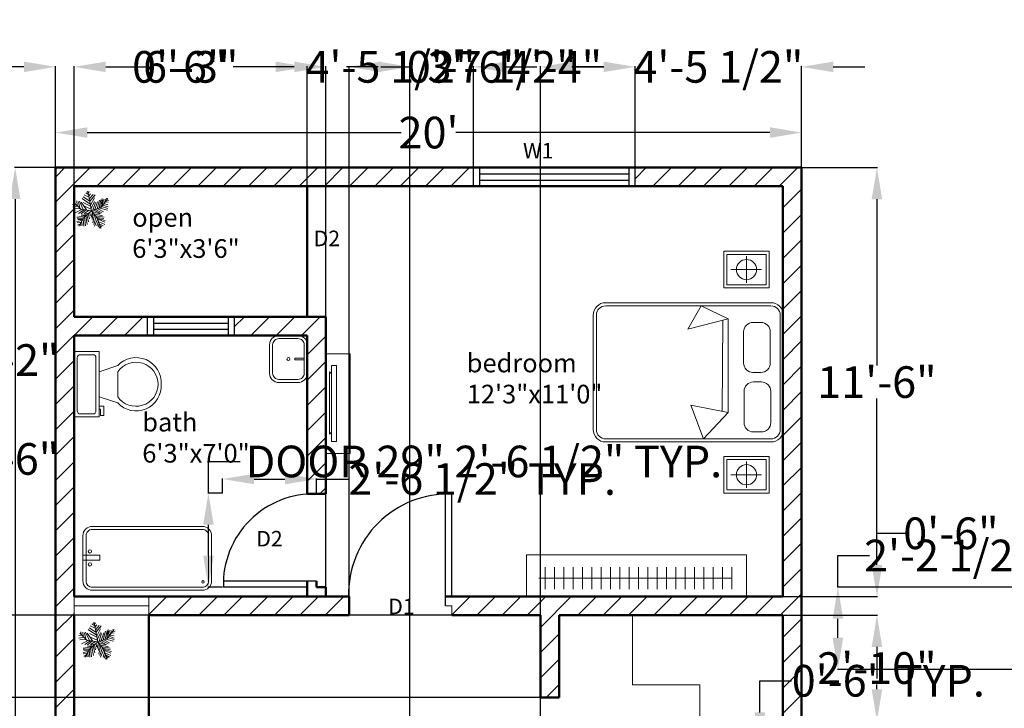
# Model space of a CAD drawing. Units: inches. Extents: x 21 to 3450, y 4 to 2137.
# Tile 11 of 14: x 2805 to 3122, y 1333 to 1554. Entities that reach past the tile are written whole.
import ezdxf

# ---------------------------------------------------------------- set-up
doc = ezdxf.new("R2010")
doc.units = ezdxf.units.IN
doc.header["$MEASUREMENT"] = 0
for name, color, linetype, lineweight in [('A-ANNO-DIMS', 2, 'Continuous', 18), ('A-ANNO-TEXT', 7, 'Continuous', 18), ('A-AREA-IDEN', 3, 'Continuous', 18), ('A-DOOR', 4, 'Continuous', 25), ('A-FLOR-FIXT', 9, 'Continuous', 18), ('A-FURN', 8, 'Continuous', 18), ('A-GLAZ', 3, 'Continuous', 25), ('A-WALL', 7, 'Continuous', 50), ('A-WALL-PATT', 8, 'Continuous', 13), ('L-PLNT', 94, 'Continuous', 13)]:
    doc.layers.add(name, color=color, linetype=linetype, lineweight=lineweight)
doc.styles.get("Standard").update_dxf_attribs({"font": 'arial.ttf'})
doc.dimstyles.get("Standard").update_dxf_attribs({"dimtxt": 10.18, "dimasz": 10.18, "dimexe": 0.18, "dimexo": 0.0625, "dimgap": 0.09, "dimtad": 0, "dimtih": 1, "dimtoh": 1, "dimdec": 0, "dimzin": 0, "dimdsep": 46, "dimlunit": 3, "dimtxsty": 'Standard', "dimcen": 0.09, "dimadec": 0, "dimazin": 0, "dimtfac": 1, "dimtdec": 0, "dimtofl": 0, "dimtmove": 0, "dimatfit": 3, "dimfxl": 1, "dimtolj": 1, "dimtzin": 0, "dimarcsym": 0})

# ---------------------------------------------------------------- blocks, each defined once
blk = doc.blocks.new('*U4')
for p, q in [((9.5, -6), (9.5, -2)), ((-10, -8.5), (-8, -8.5)), ((-10, -9.5), (-10, -8.5)), ((-7, -9.5), (-10, -9.5)), ((-8, -8.5), (-8, -8)), ((-7, -8), (-7, -9.5)), ((-4, -8), (-6, -14)), ((4, -8), (6, -14)), ((4, -14), (-4, -14))]:
    blk.add_line(p, q)
blk.add_lwpolyline([(10.5, -8), (10.5, 0), (-10.5, 0), (-10.5, -8)], close=True)
for points in [[(-9.5, -2), (-9.5, -6)], [(8.5, -1), (-8.5, -1)], [(-8.5, -7), (8.5, -7)]]:
    blk.add_lwpolyline(points)
for centre, radius, start, end in [((-8.625, -1.875), 0.8839, 81.8699, 188.1301), ((8.625, -1.875), 0.8839, 351.8699, 98.1301), ((-8.625, -6.125), 0.8839, 171.869898, 278.1301), ((8.625, -6.125), 0.8839, 261.8699, 8.1301), ((-0.4772, -19.9188), 8.0953, 133.01722, 273.38), ((0.0374, -19.8731), 7.127, 124.50543, 269.7), ((-0.0373, -19.8731), 7.127, 270.3, 55.4946), ((0.4773, -19.9188), 8.0953, 266.62, 46.9828)]:
    blk.add_arc(centre, radius, start, end)
blk = doc.blocks.new('*U6')
for p, q in [((-48.585, 21.131), (-49.309, 29.026)), ((-3.665, 19.273), (-27.574, 35.527)), ((-5.114, 28.097), (-24.676, 40.636)), ((-7.288, 39.707), (-21.778, 46.673)), ((-8.737, 47.138), (-17.069, 52.711)), ((-10.186, 53.64), (-13.084, 55.962)), ((0, 0), (-10.5, 57)), ((-9.099, 51.782), (-6.563, 55.962)), ((-7.65, 43.423), (-2.578, 49.46)), ((-5.839, 35.992), (4.667, 48.067)), ((-5.114, 27.632), (10.463, 46.673)), ((-2.941, 16.486), (8.652, 37.85)), ((16.259, 5.805), (23.142, 31.348)), ((22.055, 7.198), (27.489, 32.277)), ((27, 9), (48, 36)), ((27.127, 9.056), (31.112, 35.992)), ((31.836, 30.883), (32.561, 16.486)), ((35.096, 32.741), (37.27, 22.524)), ((38.719, 34.134), (41.979, 28.561)), ((43.791, 29.954), (51.036, 30.883)), ((44.153, 36.456), (45.239, 32.741)), ((-47.498, 19.737), (-55.83, 18.344)), ((-40.615, 13.7), (-55.105, 10.913)), ((-31.5, 4.5), (-52.5, 25.5)), ((-33.37, 6.269), (-52.207, 5.34)), ((-28.299, 3.483), (-47.86, -5.805)), ((-43.513, 28.561), (-42.427, 15.558)), ((-38.442, 26.239), (-34.819, 7.663)), ((-21.416, 3.018), (-38.079, -8.128)), ((-35.544, 28.097), (-24.314, 3.947)), ((0, 0), (-31.5, 4.5)), ((-14.533, 2.09), (-30.834, 25.31)), ((-15.982, 2.09), (-30.11, -9.521)), ((-24.314, 23.917), (-2.941, 13.7)), ((0, 0), (-22.5, -19.5)), ((-6.563, 1.161), (-21.416, -8.128)), ((-20.691, 13.7), (-1.129, 4.876)), ((-1.129, 6.734), (9.014, 26.704)), ((0, 0), (27, 9)), ((0, 0), (18, -22.5)), ((3.942, 1.625), (11.187, 24.381)), ((6.478, 1.625), (26.04, -8.592)), ((10.101, 3.483), (17.708, 26.239)), ((11.187, 3.483), (30.749, -5.805)), ((18.07, 5.805), (35.096, -3.483)), ((24.229, 7.663), (46.688, 1.625)), ((29.662, 12.307), (48.137, 6.269)), ((33.285, 16.486), (48.862, 10.913)), ((36.183, 19.737), (48.137, 17.88)), ((40.53, 25.775), (48.862, 24.846)), ((-17.431, -15.094), (-42.789, -18.809)), ((-24.314, -21.596), (-42.427, -22.06)), ((-26.849, -26.24), (-40.253, -25.775)), ((-22.5, -19.5), (-37.5, -45)), ((-15.257, -12.772), (-30.11, -12.772)), ((-25.038, -23.918), (-22.865, -45.281)), ((-20.691, -18.345), (-17.793, -44.352)), ((-6.563, -5.805), (-19.967, -9.985)), ((-17.069, -15.094), (-12.721, -40.172)), ((-13.446, -11.378), (-8.737, -32.741)), ((-9.461, -8.592), (-6.201, -23.453)), ((-4.752, -3.483), (-3.665, -14.629)), ((2.493, -3.019), (-1.491, -20.202)), ((1.769, -2.555), (24.229, -9.521)), ((5.029, -6.27), (2.131, -25.775)), ((9.014, -11.378), (3.58, -35.992)), ((14.085, -16.951), (6.478, -40.172)), ((7.565, -9.056), (32.198, -14.629)), ((18.07, -22.524), (8.289, -45.745)), ((12.274, -15.094), (36.907, -18.809)), ((16.259, -19.738), (36.183, -22.989)), ((18, -22.5), (27, -52.5)), ((18.433, -22.524), (40.53, -29.026)), ((19.157, -25.311), (38.719, -33.206)), ((-28.299, -29.026), (-42.789, -31.348)), ((-30.834, -34.135), (-42.427, -35.528)), ((-34.457, -39.708), (-40.978, -42.494)), ((-32.646, -36.921), (-31.921, -44.352)), ((-29.023, -30.884), (-27.936, -43.887)), ((20.244, -30.419), (15.897, -44.816)), ((22.78, -37.85), (19.519, -48.532)), ((21.331, -32.741), (39.081, -40.636)), ((22.78, -38.314), (34.372, -44.816)), ((24.591, -45.745), (23.142, -50.854)), ((24.591, -43.423), (30.749, -47.603)), ((26.764, -49.925), (28.213, -50.854))]:
    blk.add_line(p, q)
blk = doc.blocks.new('*D7')
at = {"layer": 'A-ANNO-DIMS', "color": 0, "lineweight": -2, "transparency": 16777216}
for p, q in [((2816.91, 1506.81), (2816.91, 1518.2)), ((2827.09, 1518.02), (2928.1, 1518.02)), ((3046.73, 1518.02), (2945.73, 1518.02)), ((3056.91, 1506.81), (3056.91, 1518.2))]:
    blk.add_line(p, q, dxfattribs=at)
at = {"layer": 'A-ANNO-DIMS', "color": 0, "transparency": 16777216}
for points in [[(2827.09, 1519.72), (2827.09, 1516.33), (2816.91, 1518.02)], [(3046.73, 1519.72), (3046.73, 1516.33), (3056.91, 1518.02)]]:
    blk.add_solid(points, dxfattribs=at)
at = {"layer": 'Defpoints', "color": 0, "transparency": 16777216}
for p in [(3056.91, 1518.02), (2816.91, 1506.74), (3056.91, 1506.74)]:
    blk.add_point(p, dxfattribs=at)
at = {"layer": 'A-ANNO-DIMS', "color": 0, "transparency": 16777216, "insert": (2936.91, 1518.02), "char_height": 10.18, "attachment_point": 5}
blk.add_mtext("\\A1;20'", dxfattribs=at)
blk = doc.blocks.new('*D8')
at = {"layer": 'A-ANNO-DIMS', "color": 0, "lineweight": -2, "transparency": 16777216}
for p, q in [((2816.85, 1506.81), (2803.73, 1506.81)), ((2803.91, 1496.63), (2803.91, 1302.07)), ((2803.91, 1096.92), (2803.91, 1291.48)), ((2999.5, 1086.74), (2803.73, 1086.74))]:
    blk.add_line(p, q, dxfattribs=at)
at = {"layer": 'A-ANNO-DIMS', "color": 0, "transparency": 16777216}
for points in [[(2802.22, 1496.63), (2805.61, 1496.63), (2803.91, 1506.81)], [(2802.22, 1096.92), (2805.61, 1096.92), (2803.91, 1086.74)]]:
    blk.add_solid(points, dxfattribs=at)
at = {"layer": 'Defpoints', "color": 0, "transparency": 16777216}
for p in [(2816.91, 1506.81), (2803.91, 1086.74), (2999.56, 1086.74)]:
    blk.add_point(p, dxfattribs=at)
at = {"layer": 'A-ANNO-DIMS', "color": 0, "transparency": 16777216, "insert": (2803.91, 1296.77), "char_height": 10.18, "attachment_point": 5}
blk.add_mtext("\\A1;35'", dxfattribs=at)
blk = doc.blocks.new('DOOR-29IN')
blk.add_line((27.01, 0), (0.01, 0))
blk.add_arc((29.01, 1), 29.02, 88.0251, 181.9749)
blk = doc.blocks.new('DOOR-32IN')
blk.add_line((33.21, 0), (33.21, 33))
blk.add_arc((32.21, 0.79), 32.22, 88.2217, 181.4078)
blk = doc.blocks.new('*D22')
at = {"layer": 'A-ANNO-DIMS', "color": 0, "lineweight": -2, "transparency": 16777216}
for p, q in [((2866.09, 1402.02), (2866.09, 1412.2)), ((2866.09, 1412.2), (2876.27, 1412.2)), ((2870.57, 1402.02), (2865.91, 1402.02)), ((2866.09, 1381.92), (2866.09, 1391.84)), ((2870.57, 1371.74), (2865.91, 1371.74))]:
    blk.add_line(p, q, dxfattribs=at)
at = {"layer": 'A-ANNO-DIMS', "color": 0, "transparency": 16777216}
for points in [[(2864.4, 1391.84), (2867.79, 1391.84), (2866.09, 1402.02)], [(2864.4, 1381.92), (2867.79, 1381.92), (2866.09, 1371.74)]]:
    blk.add_solid(points, dxfattribs=at)
at = {"layer": 'Defpoints', "color": 0, "transparency": 16777216}
for p in [(2866.09, 1402.02), (2870.63, 1402.02), (2870.63, 1371.74)]:
    blk.add_point(p, dxfattribs=at)
at = {"layer": 'A-ANNO-DIMS', "color": 0, "transparency": 16777216, "insert": (2954.71, 1412.2), "char_height": 10.18, "attachment_point": 5}
blk.add_mtext('\\A1;DOOR 29" 2\'-6 1/2" TYP.', dxfattribs=at)
blk = doc.blocks.new('*D23')
at = {"layer": 'A-ANNO-DIMS', "color": 0, "lineweight": -2, "transparency": 16777216}
for p, q in [((2870.63, 1402.08), (2870.63, 1406.74)), ((2880.81, 1406.56), (2890.73, 1406.56)), ((2900.91, 1402.08), (2900.91, 1406.74)), ((2900.91, 1406.56), (2911.09, 1406.56))]:
    blk.add_line(p, q, dxfattribs=at)
at = {"layer": 'A-ANNO-DIMS', "color": 0, "transparency": 16777216}
for points in [[(2880.81, 1408.26), (2880.81, 1404.87), (2870.63, 1406.56)], [(2890.73, 1408.26), (2890.73, 1404.87), (2900.91, 1406.56)]]:
    blk.add_solid(points, dxfattribs=at)
at = {"layer": 'Defpoints', "color": 0, "transparency": 16777216}
for p in [(2900.91, 1406.56), (2870.63, 1402.02), (2900.91, 1402.02)]:
    blk.add_point(p, dxfattribs=at)
at = {"layer": 'A-ANNO-DIMS', "color": 0, "transparency": 16777216, "insert": (2954.16, 1406.56), "char_height": 10.18, "attachment_point": 5}
blk.add_mtext('\\A1;2\'-6 1/2" TYP.', dxfattribs=at)
blk = doc.blocks.new('*D32')
at = {"layer": 'A-ANNO-DIMS', "color": 0, "lineweight": -2, "transparency": 16777216}
for p, q in [((3035.54, 1315.23), (3035.54, 1314.07)), ((3042.48, 1315.23), (3042.48, 1314.07)), ((3025.36, 1314.25), (3015.18, 1314.25)), ((3052.66, 1314.25), (3062.84, 1314.25))]:
    blk.add_line(p, q, dxfattribs=at)
at = {"layer": 'A-ANNO-DIMS', "color": 0, "transparency": 16777216}
for points in [[(3025.36, 1315.95), (3025.36, 1312.56), (3035.54, 1314.25)], [(3052.66, 1315.95), (3052.66, 1312.56), (3042.48, 1314.25)]]:
    blk.add_solid(points, dxfattribs=at)
at = {"layer": 'Defpoints', "color": 0, "transparency": 16777216}
for p in [(3035.54, 1315.29), (3042.48, 1315.29), (3042.48, 1314.25)]:
    blk.add_point(p, dxfattribs=at)
at = {"layer": 'A-ANNO-DIMS', "color": 0, "transparency": 16777216, "insert": (3152.02, 1314.25), "char_height": 10.18, "attachment_point": 5}
blk.add_mtext('\\A1;STOVE BURNER 0\'-7" TYP.', dxfattribs=at)
blk = doc.blocks.new('*D33')
at = {"layer": 'A-ANNO-DIMS', "color": 0, "lineweight": -2, "transparency": 16777216}
for p, q in [((3043.53, 1331.47), (3043.53, 1341.65)), ((3043.53, 1341.65), (3053.71, 1341.65)), ((3042.55, 1321.29), (3043.71, 1321.29)), ((3042.55, 1315.29), (3043.71, 1315.29)), ((3043.53, 1305.11), (3043.53, 1294.93))]:
    blk.add_line(p, q, dxfattribs=at)
at = {"layer": 'A-ANNO-DIMS', "color": 0, "transparency": 16777216}
for points in [[(3041.83, 1331.47), (3045.22, 1331.47), (3043.53, 1321.29)], [(3041.83, 1305.11), (3045.22, 1305.11), (3043.53, 1315.29)]]:
    blk.add_solid(points, dxfattribs=at)
at = {"layer": 'Defpoints', "color": 0, "transparency": 16777216}
for p in [(3042.48, 1321.29), (3043.53, 1321.29), (3042.48, 1315.29)]:
    blk.add_point(p, dxfattribs=at)
at = {"layer": 'A-ANNO-DIMS', "color": 0, "transparency": 16777216, "insert": (3084.82, 1341.65), "char_height": 10.18, "attachment_point": 5}
blk.add_mtext('\\A1;0\'-6" TYP.', dxfattribs=at)
blk = doc.blocks.new('*D79')
at = {"layer": 'A-ANNO-DIMS', "color": 0, "lineweight": -2, "transparency": 16777216}
for p, q in [((2778.96, 1402.83), (2778.96, 1413.01)), ((2778.96, 1413.01), (2789.14, 1413.01)), ((2749.77, 1392.65), (2779.14, 1392.65)), ((2749.77, 1386.65), (2779.14, 1386.65)), ((2778.96, 1376.47), (2778.96, 1366.29))]:
    blk.add_line(p, q, dxfattribs=at)
at = {"layer": 'A-ANNO-DIMS', "color": 0, "transparency": 16777216}
for points in [[(2777.26, 1402.83), (2780.65, 1402.83), (2778.96, 1392.65)], [(2777.26, 1376.47), (2780.65, 1376.47), (2778.96, 1386.65)]]:
    blk.add_solid(points, dxfattribs=at)
at = {"layer": 'Defpoints', "color": 0, "transparency": 16777216}
for p in [(2749.71, 1392.65), (2778.96, 1392.65), (2749.71, 1386.65)]:
    blk.add_point(p, dxfattribs=at)
at = {"layer": 'A-ANNO-DIMS', "color": 0, "transparency": 16777216, "insert": (2802.76, 1413.01), "char_height": 10.18, "attachment_point": 5}
blk.add_mtext('\\A1;0\'-6"', dxfattribs=at)
blk = doc.blocks.new('*D82')
at = {"layer": 'A-ANNO-DIMS', "color": 0, "lineweight": -2, "transparency": 16777216}
for p, q in [((2778.96, 1434.65), (2778.96, 1444.83)), ((2778.96, 1444.83), (2789.14, 1444.83)), ((2602.77, 1434.65), (2779.14, 1434.65)), ((2778.96, 1418.61), (2778.96, 1424.47)), ((2602.9, 1408.43), (2779.14, 1408.43))]:
    blk.add_line(p, q, dxfattribs=at)
at = {"layer": 'A-ANNO-DIMS', "color": 0, "transparency": 16777216}
for points in [[(2777.26, 1424.47), (2780.65, 1424.47), (2778.96, 1434.65)], [(2777.26, 1418.61), (2780.65, 1418.61), (2778.96, 1408.43)]]:
    blk.add_solid(points, dxfattribs=at)
at = {"layer": 'Defpoints', "color": 0, "transparency": 16777216}
for p in [(2602.71, 1434.65), (2778.96, 1434.65), (2602.84, 1408.43)]:
    blk.add_point(p, dxfattribs=at)
at = {"layer": 'A-ANNO-DIMS', "color": 0, "transparency": 16777216, "insert": (2802.84, 1444.83), "char_height": 10.18, "attachment_point": 5}
blk.add_mtext('\\A1;2\'-2"', dxfattribs=at)
blk = doc.blocks.new('*D96')
at = {"layer": 'A-ANNO-DIMS', "color": 0, "lineweight": -2, "transparency": 16777216}
for p, q in [((2806.73, 1539.16), (2796.55, 1539.16)), ((2816.91, 1506.81), (2816.91, 1539.34)), ((2822.91, 1500.81), (2822.91, 1539.34)), ((2833.09, 1539.16), (2843.27, 1539.16))]:
    blk.add_line(p, q, dxfattribs=at)
at = {"layer": 'A-ANNO-DIMS', "color": 0, "transparency": 16777216}
for points in [[(2806.73, 1540.85), (2806.73, 1537.46), (2816.91, 1539.16)], [(2833.09, 1540.85), (2833.09, 1537.46), (2822.91, 1539.16)]]:
    blk.add_solid(points, dxfattribs=at)
at = {"layer": 'Defpoints', "color": 0, "transparency": 16777216}
for p in [(2822.91, 1539.16), (2816.91, 1506.74), (2822.91, 1500.74)]:
    blk.add_point(p, dxfattribs=at)
at = {"layer": 'A-ANNO-DIMS', "color": 0, "transparency": 16777216, "insert": (2856.89, 1539.16), "char_height": 10.18, "attachment_point": 5}
blk.add_mtext('\\A1;0\'-6"', dxfattribs=at)
blk = doc.blocks.new('*D97')
at = {"layer": 'A-ANNO-DIMS', "color": 0, "lineweight": -2, "transparency": 16777216}
for p, q in [((2822.91, 1500.81), (2822.91, 1539.34)), ((2833.09, 1539.16), (2846.76, 1539.16)), ((2887.73, 1539.16), (2874.06, 1539.16)), ((2897.91, 1500.81), (2897.91, 1539.34))]:
    blk.add_line(p, q, dxfattribs=at)
at = {"layer": 'A-ANNO-DIMS', "color": 0, "transparency": 16777216}
for points in [[(2833.09, 1540.85), (2833.09, 1537.46), (2822.91, 1539.16)], [(2887.73, 1540.85), (2887.73, 1537.46), (2897.91, 1539.16)]]:
    blk.add_solid(points, dxfattribs=at)
at = {"layer": 'Defpoints', "color": 0, "transparency": 16777216}
for p in [(2897.91, 1539.16), (2822.91, 1500.74), (2897.91, 1500.74)]:
    blk.add_point(p, dxfattribs=at)
at = {"layer": 'A-ANNO-DIMS', "color": 0, "transparency": 16777216, "insert": (2860.41, 1539.16), "char_height": 10.18, "attachment_point": 5}
blk.add_mtext('\\A1;6\'-3"', dxfattribs=at)
blk = doc.blocks.new('*D98')
at = {"layer": 'A-ANNO-DIMS', "color": 0, "lineweight": -2, "transparency": 16777216}
for p, q in [((2887.73, 1539.16), (2877.55, 1539.16)), ((2897.91, 1500.81), (2897.91, 1539.34)), ((2951.41, 1506.81), (2951.41, 1539.34)), ((2961.59, 1539.16), (2971.77, 1539.16))]:
    blk.add_line(p, q, dxfattribs=at)
at = {"layer": 'A-ANNO-DIMS', "color": 0, "transparency": 16777216}
for points in [[(2887.73, 1540.85), (2887.73, 1537.46), (2897.91, 1539.16)], [(2961.59, 1540.85), (2961.59, 1537.46), (2951.41, 1539.16)]]:
    blk.add_solid(points, dxfattribs=at)
at = {"layer": 'Defpoints', "color": 0, "transparency": 16777216}
for p in [(2951.41, 1539.16), (2951.41, 1506.74), (2897.91, 1500.74)]:
    blk.add_point(p, dxfattribs=at)
at = {"layer": 'A-ANNO-DIMS', "color": 0, "transparency": 16777216, "insert": (2924.66, 1539.16), "char_height": 10.18, "attachment_point": 5}
blk.add_mtext('\\A1;4\'-5 1/2"', dxfattribs=at)
blk = doc.blocks.new('*D99')
at = {"layer": 'A-ANNO-DIMS', "color": 0, "lineweight": -2, "transparency": 16777216}
for p, q in [((2951.41, 1506.81), (2951.41, 1539.34)), ((2961.59, 1539.16), (2963.59, 1539.16)), ((2993.23, 1539.16), (2991.24, 1539.16)), ((3003.41, 1506.81), (3003.41, 1539.34))]:
    blk.add_line(p, q, dxfattribs=at)
at = {"layer": 'A-ANNO-DIMS', "color": 0, "transparency": 16777216}
for points in [[(2961.59, 1540.85), (2961.59, 1537.46), (2951.41, 1539.16)], [(2993.23, 1540.85), (2993.23, 1537.46), (3003.41, 1539.16)]]:
    blk.add_solid(points, dxfattribs=at)
at = {"layer": 'Defpoints', "color": 0, "transparency": 16777216}
for p in [(3003.41, 1539.16), (2951.41, 1506.74), (3003.41, 1506.74)]:
    blk.add_point(p, dxfattribs=at)
at = {"layer": 'A-ANNO-DIMS', "color": 0, "transparency": 16777216, "insert": (2977.41, 1539.16), "char_height": 10.18, "attachment_point": 5}
blk.add_mtext('\\A1;4\'-4"', dxfattribs=at)
blk = doc.blocks.new('*D100')
at = {"layer": 'A-ANNO-DIMS', "color": 0, "lineweight": -2, "transparency": 16777216}
for p, q in [((2993.23, 1539.16), (2983.05, 1539.16)), ((3003.41, 1506.81), (3003.41, 1539.34)), ((3056.91, 1506.81), (3056.91, 1539.34)), ((3067.09, 1539.16), (3077.27, 1539.16))]:
    blk.add_line(p, q, dxfattribs=at)
at = {"layer": 'A-ANNO-DIMS', "color": 0, "transparency": 16777216}
for points in [[(2993.23, 1540.85), (2993.23, 1537.46), (3003.41, 1539.16)], [(3067.09, 1540.85), (3067.09, 1537.46), (3056.91, 1539.16)]]:
    blk.add_solid(points, dxfattribs=at)
at = {"layer": 'Defpoints', "color": 0, "transparency": 16777216}
for p in [(3056.91, 1539.16), (3003.41, 1506.74), (3056.91, 1506.74)]:
    blk.add_point(p, dxfattribs=at)
at = {"layer": 'A-ANNO-DIMS', "color": 0, "transparency": 16777216, "insert": (3030.16, 1539.16), "char_height": 10.18, "attachment_point": 5}
blk.add_mtext('\\A1;4\'-5 1/2"', dxfattribs=at)
blk = doc.blocks.new('*D111')
at = {"layer": 'A-ANNO-DIMS', "color": 0, "lineweight": -2, "transparency": 16777216}
for p, q in [((3050.97, 1362.74), (3081.34, 1362.74)), ((3081.16, 1352.56), (3081.16, 1351.03)), ((3081.16, 1338.92), (3081.16, 1340.46)), ((3056.97, 1328.74), (3081.34, 1328.74))]:
    blk.add_line(p, q, dxfattribs=at)
at = {"layer": 'A-ANNO-DIMS', "color": 0, "transparency": 16777216}
for points in [[(3079.47, 1352.56), (3082.86, 1352.56), (3081.16, 1362.74)], [(3079.47, 1338.92), (3082.86, 1338.92), (3081.16, 1328.74)]]:
    blk.add_solid(points, dxfattribs=at)
at = {"layer": 'Defpoints', "color": 0, "transparency": 16777216}
for p in [(3050.91, 1362.74), (3081.16, 1362.74), (3056.91, 1328.74)]:
    blk.add_point(p, dxfattribs=at)
at = {"layer": 'A-ANNO-DIMS', "color": 0, "transparency": 16777216, "insert": (3081.16, 1345.74), "char_height": 10.18, "attachment_point": 5}
blk.add_mtext('\\A1;2\'-10"', dxfattribs=at)
blk = doc.blocks.new('*D112')
at = {"layer": 'A-ANNO-DIMS', "color": 0, "lineweight": -2, "transparency": 16777216}
for p, q in [((3081.16, 1378.92), (3081.16, 1389.1)), ((3081.16, 1389.1), (3091.34, 1389.1)), ((3050.97, 1368.74), (3081.34, 1368.74)), ((3050.97, 1362.74), (3081.34, 1362.74)), ((3081.16, 1352.56), (3081.16, 1342.38))]:
    blk.add_line(p, q, dxfattribs=at)
at = {"layer": 'A-ANNO-DIMS', "color": 0, "transparency": 16777216}
for points in [[(3079.47, 1378.92), (3082.86, 1378.92), (3081.16, 1368.74)], [(3079.47, 1352.56), (3082.86, 1352.56), (3081.16, 1362.74)]]:
    blk.add_solid(points, dxfattribs=at)
at = {"layer": 'Defpoints', "color": 0, "transparency": 16777216}
for p in [(3050.91, 1368.74), (3081.16, 1368.74), (3050.91, 1362.74)]:
    blk.add_point(p, dxfattribs=at)
at = {"layer": 'A-ANNO-DIMS', "color": 0, "transparency": 16777216, "insert": (3104.96, 1389.1), "char_height": 10.18, "attachment_point": 5}
blk.add_mtext('\\A1;0\'-6"', dxfattribs=at)
blk = doc.blocks.new('*D113')
at = {"layer": 'A-ANNO-DIMS', "color": 0, "lineweight": -2, "transparency": 16777216}
for p, q in [((3056.97, 1506.74), (3081.34, 1506.74)), ((3081.16, 1496.56), (3081.16, 1443.03)), ((3081.16, 1378.92), (3081.16, 1432.46)), ((3050.97, 1368.74), (3081.34, 1368.74))]:
    blk.add_line(p, q, dxfattribs=at)
at = {"layer": 'A-ANNO-DIMS', "color": 0, "transparency": 16777216}
for points in [[(3079.47, 1496.56), (3082.86, 1496.56), (3081.16, 1506.74)], [(3079.47, 1378.92), (3082.86, 1378.92), (3081.16, 1368.74)]]:
    blk.add_solid(points, dxfattribs=at)
at = {"layer": 'Defpoints', "color": 0, "transparency": 16777216}
for p in [(3056.91, 1506.74), (3081.16, 1506.74), (3050.91, 1368.74)]:
    blk.add_point(p, dxfattribs=at)
at = {"layer": 'A-ANNO-DIMS', "color": 0, "transparency": 16777216, "insert": (3081.16, 1437.74), "char_height": 10.18, "attachment_point": 5}
blk.add_mtext('\\A1;11\'-6"', dxfattribs=at)
blk = doc.blocks.new('*D116')
at = {"layer": 'A-ANNO-DIMS', "color": 0, "lineweight": -2, "transparency": 16777216}
for p, q in [((2893.73, 1539.16), (2883.55, 1539.16)), ((2903.91, 1368.81), (2903.91, 1539.34)), ((2911.4, 1368.81), (2911.4, 1539.34)), ((2921.58, 1539.16), (2931.76, 1539.16))]:
    blk.add_line(p, q, dxfattribs=at)
at = {"layer": 'A-ANNO-DIMS', "color": 0, "transparency": 16777216}
for points in [[(2893.73, 1540.85), (2893.73, 1537.46), (2903.91, 1539.16)], [(2921.58, 1540.85), (2921.58, 1537.46), (2911.4, 1539.16)]]:
    blk.add_solid(points, dxfattribs=at)
at = {"layer": 'Defpoints', "color": 0, "transparency": 16777216}
for p in [(2911.4, 1539.16), (2903.91, 1368.74), (2911.4, 1368.74)]:
    blk.add_point(p, dxfattribs=at)
at = {"layer": 'A-ANNO-DIMS', "color": 0, "transparency": 16777216, "insert": (2957.24, 1539.16), "char_height": 10.18, "attachment_point": 5}
blk.add_mtext('\\A1;0\'-7 1/2"', dxfattribs=at)
blk = doc.blocks.new('*D118')
at = {"layer": 'A-ANNO-DIMS', "color": 0, "lineweight": -2, "transparency": 16777216}
for p, q in [((2920.73, 1539.16), (2910.55, 1539.16)), ((2930.91, 1242.81), (2930.91, 1539.34)), ((2972.91, 1242.81), (2972.91, 1539.34)), ((2983.09, 1539.16), (2993.27, 1539.16))]:
    blk.add_line(p, q, dxfattribs=at)
at = {"layer": 'A-ANNO-DIMS', "color": 0, "transparency": 16777216}
for points in [[(2920.73, 1540.85), (2920.73, 1537.46), (2930.91, 1539.16)], [(2983.09, 1540.85), (2983.09, 1537.46), (2972.91, 1539.16)]]:
    blk.add_solid(points, dxfattribs=at)
at = {"layer": 'Defpoints', "color": 0, "transparency": 16777216}
for p in [(2972.91, 1539.16), (2930.91, 1242.74), (2972.91, 1242.74)]:
    blk.add_point(p, dxfattribs=at)
at = {"layer": 'A-ANNO-DIMS', "color": 0, "transparency": 16777216, "insert": (2951.91, 1539.16), "char_height": 10.18, "attachment_point": 5}
blk.add_mtext('\\A1;3\'-6"', dxfattribs=at)
blk = doc.blocks.new('*D119')
at = {"layer": 'A-ANNO-DIMS', "color": 0, "lineweight": -2, "transparency": 16777216}
for p, q in [((2738.66, 1362.74), (2738.66, 1372.92)), ((2738.66, 1372.92), (2748.84, 1372.92)), ((2972.85, 1362.74), (2738.48, 1362.74)), ((2738.66, 1346.47), (2738.66, 1352.56)), ((2972.85, 1336.29), (2738.48, 1336.29))]:
    blk.add_line(p, q, dxfattribs=at)
at = {"layer": 'A-ANNO-DIMS', "color": 0, "transparency": 16777216}
for points in [[(2736.97, 1352.56), (2740.36, 1352.56), (2738.66, 1362.74)], [(2736.97, 1346.47), (2740.36, 1346.47), (2738.66, 1336.29)]]:
    blk.add_solid(points, dxfattribs=at)
at = {"layer": 'Defpoints', "color": 0, "transparency": 16777216}
for p in [(2738.66, 1362.74), (2972.91, 1362.74), (2972.91, 1336.29)]:
    blk.add_point(p, dxfattribs=at)
at = {"layer": 'A-ANNO-DIMS', "color": 0, "transparency": 16777216, "insert": (2774.41, 1372.92), "char_height": 10.18, "attachment_point": 5}
blk.add_mtext('\\A1;2\'-2 1/2"', dxfattribs=at)
blk = doc.blocks.new('*D146')
at = {"layer": 'A-ANNO-DIMS', "color": 0, "lineweight": -2, "transparency": 16777216}
for p, q in [((3068.61, 1371.77), (3068.61, 1381.95)), ((3068.61, 1381.95), (3078.79, 1381.95)), ((3302.55, 1371.77), (3068.43, 1371.77)), ((3068.61, 1355.5), (3068.61, 1361.59)), ((3302.55, 1345.32), (3068.43, 1345.32))]:
    blk.add_line(p, q, dxfattribs=at)
at = {"layer": 'A-ANNO-DIMS', "color": 0, "transparency": 16777216}
for points in [[(3066.91, 1361.59), (3070.31, 1361.59), (3068.61, 1371.77)], [(3066.91, 1355.5), (3070.31, 1355.5), (3068.61, 1345.32)]]:
    blk.add_solid(points, dxfattribs=at)
at = {"layer": 'Defpoints', "color": 0, "transparency": 16777216}
for p in [(3068.61, 1371.77), (3302.61, 1371.77), (3302.61, 1345.32)]:
    blk.add_point(p, dxfattribs=at)
at = {"layer": 'A-ANNO-DIMS', "color": 0, "transparency": 16777216, "insert": (3104.36, 1381.95), "char_height": 10.18, "attachment_point": 5}
blk.add_mtext('\\A1;2\'-2 1/2"', dxfattribs=at)

msp = doc.modelspace()

# ---------------------------------------------------------------- hatches: boundary and pattern name
at = {"layer": 'A-WALL-PATT'}
h = msp.add_hatch(dxfattribs=at)
h.set_pattern_fill('ANSI31', color=256, scale=46)
h.set_pattern_definition([(45, (-32.016, 151.0237), (-4.065864, 4.065864), [])])
h.paths.add_polyline_path([(2951.41, 1506.74), (2816.91, 1506.74), (2816.91, 1190.74), (2822.91, 1190.74), (2822.91, 1236.74), (2822.91, 1242.74), (2822.91, 1362.74), (2822.91, 1368.74), (2822.91, 1452.74), (2846.41, 1452.74), (2846.41, 1458.74), (2822.91, 1458.74), (2822.91, 1500.74), (2897.91, 1500.74), (2903.91, 1500.74), (2951.41, 1500.74)])
h.paths.add_polyline_path([(3056.91, 1506.74), (3003.41, 1506.74), (3003.41, 1500.74), (3050.91, 1500.74), (3050.91, 1460.31, -0.065004), (3051.05, 1459.28), (3051.05, 1422.47, -0.065004), (3050.91, 1421.45), (3050.91, 1368.74), (2942.4, 1368.74), (2942.4, 1365.74), (2944.4, 1365.74), (2944.4, 1362.74), (2972.91, 1362.74), (2972.91, 1336.29), (2978.91, 1336.29), (2978.91, 1362.74), (3050.91, 1362.74), (3050.91, 1328.74), (3056.91, 1328.74)])
h.paths.add_polyline_path([(2885.91, 1239.74), (2885.91, 1242.74), (2852.91, 1242.74), (2852.91, 1324.17), (2846.91, 1324.17), (2846.91, 1242.74), (2846.91, 1236.74), (2885.91, 1236.74), (2885.91, 1237.74, -0.014283)], flags=17)
h.paths.add_polyline_path([(2847.91, 1092.74), (2822.91, 1092.74), (2822.91, 1138.74), (2816.91, 1138.74), (2816.91, 1086.74), (2847.91, 1086.74)])
h.paths.add_polyline_path([(2911.4, 1368.74), (2903.91, 1368.74), (2897.91, 1368.74), (2846.91, 1368.74), (2846.91, 1362.74), (2852.91, 1362.74), (2903.91, 1362.74), (2911.4, 1362.74)], flags=17)
h.paths.add_polyline_path([(2903.91, 1458.74), (2897.91, 1458.74), (2874.41, 1458.74), (2874.41, 1452.74), (2897.91, 1452.74), (2897.91, 1401.74), (2898.91, 1401.74, -0.017236), (2900.91, 1401.74), (2903.91, 1401.74), (2903.91, 1452.74)], flags=17)

# ---------------------------------------------------------------- linework, layer by layer
at = {"layer": 'A-DOOR'}
for p, q in [((2942.4, 1365.74), (2942.4, 1401.74)), ((2900.91, 1373.74), (2870.91, 1373.74))]:
    msp.add_line(p, q, dxfattribs=at)
at = {"layer": 'A-FLOR-FIXT'}
for p, q in [((2822.91, 1368.74), (2822.91, 1362.74)), ((2846.91, 1362.74), (2846.91, 1368.74)), ((2846.91, 1365.74), (2822.91, 1365.74)), ((2822.91, 1362.74), (2846.91, 1362.74)), ((3024.16, 1242.74), (3024.16, 1340.31))]:
    msp.add_line(p, q, dxfattribs=at)
for points in [[(2828.72, 1370.76, -0.414214), (2825.72, 1373.76), (2825.72, 1388.31, -0.414214), (2828.72, 1391.31), (2864.13, 1391.31, -0.414214), (2867.13, 1388.31), (2867.13, 1373.76, -0.414214), (2864.13, 1370.76)], [(2828.72, 1371.76, -0.414214), (2826.72, 1373.76), (2826.72, 1388.31, -0.414214), (2828.72, 1390.31), (2864.13, 1390.31, -0.414214), (2866.13, 1388.31), (2866.13, 1373.76, -0.414214), (2864.13, 1371.76)]]:
    msp.add_lwpolyline(points, format="xyb", close=True, dxfattribs=at)
msp.add_lwpolyline([(2825.72, 1382.05), (2825.72, 1382.05), (2831.16, 1382.05), (2831.16, 1382.05), (2831.16, 1380.46), (2831.16, 1380.46), (2825.72, 1380.46), (2825.72, 1380.46)], close=True, dxfattribs=at)
for centre, radius in [((2827.98, 1383.26), 0.546), ((2827.98, 1379.09), 0.546), ((2864.35, 1373.46), 0.395)]:
    msp.add_circle(centre, radius, dxfattribs=at)
at = {"layer": 'A-FURN'}
for p, q in [((3039.2, 1478.22), (3039.2, 1469.68)), ((3034.11, 1473.94), (3044.05, 1473.94)), ((3024.64, 1462.28), (3020.32, 1454.81)), ((3033.35, 1458.1), (3024.64, 1462.28)), ((3020.32, 1454.81), (3033.35, 1458.1)), ((3031.55, 1457.64), (3031.33, 1428.41)), ((3033.35, 1458.1), (3033.35, 1428.01)), ((2905.74, 1440.44), (2905.07, 1441.07)), ((2905.07, 1441.07), (2905.07, 1421)), ((3025.38, 1419.47), (3021.31, 1430.37)), ((3021.31, 1430.37), (3033.35, 1428.01)), ((3033.35, 1428.01), (3025.38, 1419.47)), ((2905.07, 1421), (2905.74, 1421.66)), ((3039.2, 1412.22), (3039.2, 1403.68)), ((3034.11, 1407.93), (3044.05, 1407.93)), ((2974.48, 1378.24), (2974.48, 1371.15)), ((2977.48, 1378.24), (2977.48, 1371.15)), ((2980.48, 1378.24), (2980.48, 1371.15)), ((2983.48, 1378.24), (2983.48, 1371.15)), ((2986.48, 1378.24), (2986.48, 1371.15)), ((2989.48, 1378.24), (2989.48, 1371.15)), ((2992.48, 1378.24), (2992.48, 1371.15)), ((2995.48, 1378.24), (2995.48, 1371.15)), ((2998.48, 1378.24), (2998.48, 1371.15)), ((3001.48, 1378.24), (3001.48, 1371.15)), ((3004.48, 1378.24), (3004.48, 1371.15)), ((3007.48, 1378.24), (3007.48, 1371.15)), ((3010.48, 1378.24), (3010.48, 1371.15)), ((3013.48, 1378.24), (3013.48, 1371.15)), ((3016.48, 1378.24), (3016.48, 1371.15)), ((3019.48, 1378.24), (3019.48, 1371.15)), ((3022.48, 1378.24), (3022.48, 1371.15)), ((3025.48, 1378.24), (3025.48, 1371.15)), ((3028.48, 1378.24), (3028.48, 1371.15)), ((3031.48, 1378.24), (3031.48, 1371.15)), ((3034.48, 1378.24), (3034.48, 1371.15)), ((2972.4, 1374.62), (3034.47, 1374.62)), ((2942.4, 1365.74), (2944.4, 1365.74)), ((2944.4, 1365.74), (2944.4, 1362.74)), ((3002.54, 1340.31), (3002.54, 1362.74)), ((3024.16, 1340.31), (3002.54, 1340.31))]:
    msp.add_line(p, q, dxfattribs=at)
for points in [[(3031.89, 1479.83), (3031.89, 1479.83), (3046.5, 1479.83), (3046.5, 1479.83), (3046.5, 1468.04), (3046.5, 1468.04), (3031.89, 1468.04), (3031.89, 1468.04)], [(3032.89, 1478.83), (3045.5, 1478.83), (3045.5, 1469.04), (3032.89, 1469.04)], [(2896.91, 1445.41), (2896.91, 1445.41), (2893.91, 1445.41), (2893.91, 1445.41), (2893.91, 1444.88), (2893.91, 1444.88), (2896.91, 1444.88), (2896.91, 1444.88)], [(2903.91, 1446.87), (2903.91, 1446.87), (2911.74, 1446.87), (2911.74, 1446.87), (2911.74, 1414.75), (2911.74, 1414.75), (2903.91, 1414.75), (2903.91, 1414.75)], [(2905.74, 1443.04), (2905.74, 1443.04), (2907.35, 1443.04), (2907.35, 1443.04), (2907.35, 1418.58), (2907.35, 1418.58), (2905.74, 1418.58), (2905.74, 1418.58)], [(3031.89, 1413.82), (3031.89, 1413.82), (3046.5, 1413.82), (3046.5, 1413.82), (3046.5, 1402.04), (3046.5, 1402.04), (3031.89, 1402.04), (3031.89, 1402.04)], [(3032.89, 1412.82), (3045.5, 1412.82), (3045.5, 1403.04), (3032.89, 1403.04)], [(3039.2, 1368.74), (3039.2, 1368.74), (2968.44, 1368.74), (2968.44, 1368.74), (2968.44, 1382.17), (2968.44, 1382.17), (3039.2, 1382.17), (3039.2, 1382.17)]]:
    msp.add_lwpolyline(points, close=True, dxfattribs=at)
for points in [[(3051.05, 1459.28, 0.414214), (3047.05, 1463.28), (2993.92, 1463.28, 0.414214), (2989.92, 1459.28), (2989.92, 1422.47, 0.414214), (2993.92, 1418.47), (3047.05, 1418.47, 0.414214), (3051.05, 1422.47)], [(3050.05, 1459.28, 0.414214), (3047.05, 1462.28), (2993.92, 1462.28, 0.414214), (2990.92, 1459.28), (2990.92, 1422.47, 0.414214), (2993.92, 1419.47), (3047.05, 1419.47, 0.414214), (3050.05, 1422.47)], [(3038.28, 1453.92, -0.414214), (3041.28, 1456.92), (3043.86, 1456.92, -0.414214), (3046.86, 1453.92), (3046.86, 1443.85, -0.414214), (3043.86, 1440.85), (3041.28, 1440.85, -0.414214), (3038.28, 1443.85)], [(2897.91, 1449.74, 0.414214), (2894.91, 1452.74), (2888.75, 1452.74, 0.414214), (2885.75, 1449.74), (2885.75, 1440.6, 0.414214), (2888.75, 1437.6), (2894.91, 1437.6, 0.414214), (2897.91, 1440.6)], [(2896.91, 1449.74, 0.414214), (2894.91, 1451.74), (2888.75, 1451.74, 0.414214), (2886.75, 1449.74), (2886.75, 1440.6, 0.414214), (2888.75, 1438.6), (2894.91, 1438.6, 0.414214), (2896.91, 1440.6)], [(3038.42, 1434.78, -0.414214), (3041.42, 1437.78), (3044.01, 1437.78, -0.414214), (3047.01, 1434.78), (3047.01, 1424.71, -0.414214), (3044.01, 1421.71), (3041.42, 1421.71, -0.414214), (3038.42, 1424.71)]]:
    msp.add_lwpolyline(points, format="xyb", close=True, dxfattribs=at)
for centre, radius in [((3039.2, 1473.94), 3.25), ((2891.83, 1445.17), 0.458), ((3039.2, 1407.93), 3.25)]:
    msp.add_circle(centre, radius, dxfattribs=at)
at = {"layer": 'A-GLAZ'}
for p, q in [((2951.41, 1500.74), (2951.41, 1506.74)), ((2953.41, 1500.74), (2953.41, 1506.74)), ((2953.41, 1504.74), (3001.41, 1504.74)), ((3001.41, 1500.74), (3001.41, 1506.74)), ((3003.41, 1500.74), (3003.41, 1506.74)), ((2953.41, 1502.74), (3001.41, 1502.74)), ((2846.41, 1458.74), (2846.41, 1452.74)), ((2848.41, 1458.74), (2848.41, 1452.74)), ((2872.41, 1458.74), (2872.41, 1452.74)), ((2874.41, 1458.74), (2874.41, 1452.74)), ((2848.41, 1456.74), (2872.41, 1456.74)), ((2848.41, 1454.74), (2872.41, 1454.74))]:
    msp.add_line(p, q, dxfattribs=at)
at = {"layer": 'A-WALL'}
for p, q in [((2816.91, 1086.74), (2816.91, 1506.74)), ((2816.91, 1506.74), (3056.91, 1506.74)), ((3056.91, 1506.74), (3056.91, 1086.74)), ((2822.91, 1500.74), (2897.91, 1500.74)), ((2822.91, 1458.74), (2822.91, 1500.74)), ((2897.91, 1500.74), (2903.91, 1500.74)), ((2897.91, 1458.74), (2897.91, 1500.74)), ((2903.91, 1500.74), (3050.91, 1500.74)), ((3050.91, 1500.74), (3050.91, 1368.74)), ((2822.91, 1458.74), (2897.91, 1458.74)), ((2897.91, 1458.74), (2903.91, 1458.74)), ((2903.91, 1452.74), (2903.91, 1458.74)), ((2822.91, 1452.74), (2897.91, 1452.74)), ((2822.91, 1368.74), (2822.91, 1452.74)), ((2897.91, 1401.69), (2897.91, 1452.74)), ((2903.91, 1401.74), (2903.91, 1452.74)), ((2897.91, 1401.74), (2903.91, 1401.74)), ((2897.91, 1368.74), (2897.91, 1373.74)), ((2900.91, 1373.74), (2900.91, 1371.74)), ((2900.91, 1371.74), (2903.91, 1371.74)), ((2903.91, 1368.74), (2903.91, 1371.74)), ((2822.91, 1368.74), (2897.91, 1368.74)), ((2897.91, 1368.74), (2903.91, 1368.74)), ((2903.91, 1368.74), (2911.4, 1368.74)), ((2911.4, 1368.74), (2911.4, 1362.74)), ((2942.4, 1368.74), (3050.91, 1368.74)), ((2822.91, 1242.74), (2822.91, 1362.74)), ((2846.91, 1362.74), (2846.91, 1242.74)), ((2852.91, 1362.74), (2846.91, 1362.74)), ((2852.91, 1362.74), (2903.91, 1362.74)), ((2903.91, 1362.74), (2911.4, 1362.74)), ((2944.4, 1362.74), (2972.91, 1362.74)), ((2972.91, 1362.74), (2972.91, 1336.29)), ((2978.91, 1362.74), (2978.91, 1336.29)), ((2978.91, 1362.74), (3050.91, 1362.74)), ((3050.91, 1362.74), (3050.91, 1242.74)), ((2972.91, 1336.29), (2978.91, 1336.29))]:
    msp.add_line(p, q, dxfattribs=at)

# ---------------------------------------------------------------- block references
at = {"layer": 'A-DOOR'}
for name, p in [('DOOR-29IN', (2870.9, 1371.74)), ('DOOR-32IN', (2911.19, 1368.74))]:
    msp.add_blockref(name, p, dxfattribs=at)
at = {"layer": 'A-FLOR-FIXT', "rotation": 90}
msp.add_blockref('*U4', (2822.91, 1437.04), dxfattribs=at)
at = {"layer": 'L-PLNT', "xscale": 0.1095009231923873, "yscale": 0.1095009231923873, "zscale": 0.1095009231923873}
for p in [(2828.49, 1492.88), (2830.47, 1354.2)]:
    msp.add_blockref('*U6', p, dxfattribs=at)

# ---------------------------------------------------------------- texts
at = {"layer": 'A-ANNO-TEXT', "char_height": 5, "attachment_point": 1}
for s, insert in [('W1', (2967.3, 1514.69)), ('D2', (2899.96, 1486.47)), ('D2', (2881.5, 1389.86)), ('D1', (2923.95, 1368.07))]:
    msp.add_mtext_dynamic_manual_height_columns(s, width=14.628, gutter_width=1, heights=[0], dxfattribs=dict(at, insert=insert))
at = {"layer": 'A-AREA-IDEN', "char_height": 6, "attachment_point": 1}
for s, insert in [('open\\P6\'3"x3\'6"', (2841.59, 1493.71)), ('bedroom\\P12\'3"x11\'0"', (2949.21, 1446.88)), ('bath\\P6\'3"x7\'0"', (2844.82, 1427.85))]:
    msp.add_mtext_dynamic_manual_height_columns(s, width=84.0083, gutter_width=1, heights=[0], dxfattribs=dict(at, insert=insert))

# ---------------------------------------------------------------- dimensions: what is measured, and where the dimension line sits
at = {"layer": 'A-ANNO-DIMS'}
for base, p1, p2, override, picture, middle in [((2951.41, 1539.16), (2897.91, 1500.74), (2951.41, 1506.74), {"dimdec": 1, "dimlfac": 1, "dimrnd": 0, "dimzin": 1, "dimdsep": 46, "dimlunit": 4, "dimfrac": 2}, '*D98', (2924.66, 1539.16)), ((2911.4, 1539.16), (2903.91, 1368.74), (2911.4, 1368.74), {"dimdec": 1, "dimlfac": 1, "dimrnd": 0, "dimzin": 1, "dimdsep": 46, "dimlunit": 4, "dimfrac": 2}, '*D116', (2957.24, 1539.16)), ((3056.91, 1539.16), (3003.41, 1506.74), (3056.91, 1506.74), {"dimdec": 1, "dimlfac": 1, "dimrnd": 0, "dimzin": 1, "dimdsep": 46, "dimlunit": 4, "dimfrac": 2}, '*D100', (3030.16, 1539.16)), ((2822.91, 1539.16), (2816.91, 1506.74), (2822.91, 1500.74), {"dimdec": 1, "dimlfac": 1, "dimrnd": 0, "dimzin": 1, "dimdsep": 46, "dimlunit": 4, "dimfrac": 2}, '*D96', (2856.89, 1539.16)), ((2897.91, 1539.16), (2822.91, 1500.74), (2897.91, 1500.74), {"dimdec": 1, "dimlfac": 1, "dimrnd": 0, "dimzin": 1, "dimdsep": 46, "dimlunit": 4, "dimfrac": 2}, '*D97', (2860.41, 1539.16)), ((2972.91, 1539.16), (2930.91, 1242.74), (2972.91, 1242.74), {"dimdec": 1, "dimlfac": 1, "dimrnd": 0, "dimzin": 1, "dimdsep": 46, "dimlunit": 4, "dimfrac": 2}, '*D118', (2951.91, 1539.16)), ((3003.41, 1539.16), (2951.41, 1506.74), (3003.41, 1506.74), {"dimdec": 1, "dimlfac": 1, "dimrnd": 0, "dimzin": 1, "dimdsep": 46, "dimlunit": 4, "dimfrac": 2}, '*D99', (2977.41, 1539.16)), ((3056.91, 1518.02), (2816.91, 1506.74), (3056.91, 1506.74), {"dimclrd": 0, "dimclre": 0, "dimclrt": 0}, '*D7', (2936.91, 1518.02))]:
    dim = msp.add_linear_dim(base=base, p1=p1, p2=p2, dimstyle='Standard', override=override, dxfattribs=at)
    dim.commit()
    dim.dimension.update_dxf_attribs({"geometry": picture, "text_midpoint": middle})
for base, p1, p2, override, picture, middle in [((2803.91, 1086.74), (2816.91, 1506.81), (2999.56, 1086.74), {"dimclrd": 0, "dimclre": 0, "dimclrt": 0}, '*D8', (2803.91, 1296.77)), ((3081.16, 1506.74), (3050.91, 1368.74), (3056.91, 1506.74), {"dimdec": 1, "dimlfac": 1, "dimrnd": 0, "dimzin": 1, "dimdsep": 46, "dimlunit": 4, "dimfrac": 2}, '*D113', (3081.16, 1437.74)), ((2778.96, 1434.65), (2602.84, 1408.43), (2602.71, 1434.65), {"dimdec": 1, "dimlfac": 1, "dimrnd": 0, "dimzin": 1, "dimdsep": 46, "dimlunit": 4, "dimfrac": 2}, '*D82', (2802.84, 1444.83)), ((2778.96, 1392.65), (2749.71, 1386.65), (2749.71, 1392.65), {"dimdec": 1, "dimlfac": 1, "dimrnd": 0, "dimzin": 1, "dimdsep": 46, "dimlunit": 4, "dimfrac": 2}, '*D79', (2802.76, 1413.01)), ((3068.611, 1371.7664), (3302.611, 1345.3178), (3302.611, 1371.7664), {"dimdec": 1, "dimlfac": 1, "dimrnd": 0, "dimzin": 1, "dimdsep": 46, "dimlunit": 4, "dimfrac": 2}, '*D146', (3104.3587, 1381.9464)), ((3081.16, 1368.74), (3050.91, 1362.74), (3050.91, 1368.74), {"dimdec": 1, "dimlfac": 1, "dimrnd": 0, "dimzin": 1, "dimdsep": 46, "dimlunit": 4, "dimfrac": 2}, '*D112', (3104.96, 1389.1)), ((2738.6618, 1362.7436), (2972.9118, 1336.295), (2972.9118, 1362.7436), {"dimdec": 1, "dimlfac": 1, "dimrnd": 0, "dimzin": 1, "dimdsep": 46, "dimlunit": 4, "dimfrac": 2}, '*D119', (2774.4096, 1372.9236)), ((3081.16, 1362.74), (3056.91, 1328.74), (3050.91, 1362.74), {"dimdec": 1, "dimlfac": 1, "dimrnd": 0, "dimzin": 1, "dimdsep": 46, "dimlunit": 4, "dimfrac": 2}, '*D111', (3081.16, 1345.74))]:
    dim = msp.add_linear_dim(base=base, p1=p1, p2=p2, angle=90, dimstyle='Standard', override=override, dxfattribs=at)
    dim.commit()
    dim.dimension.update_dxf_attribs({"geometry": picture, "text_midpoint": middle})
for base, p1, p2, text, picture, middle in [((2866.09, 1402.02), (2870.63, 1371.74), (2870.63, 1402.02), 'DOOR 29" <> TYP.', '*D22', (2954.71, 1412.2)), ((3043.53, 1321.29), (3042.48, 1315.29), (3042.48, 1321.29), '<> TYP.', '*D33', (3084.82, 1341.65))]:
    dim = msp.add_linear_dim(base=base, p1=p1, p2=p2, angle=90, text=text, dimstyle='Standard', override={"dimdec": 1, "dimrnd": 0, "dimzin": 1, "dimlunit": 4, "dimfrac": 2}, dxfattribs=at)
    dim.commit()
    dim.dimension.update_dxf_attribs({"geometry": picture, "text_midpoint": middle})
for base, p1, p2, text, picture, middle in [((2900.91, 1406.56), (2870.63, 1402.02), (2900.91, 1402.02), '<> TYP.', '*D23', (2954.16, 1406.56)), ((3042.48, 1314.25), (3035.54, 1315.29), (3042.48, 1315.29), 'STOVE BURNER <> TYP.', '*D32', (3152.02, 1314.25))]:
    dim = msp.add_linear_dim(base=base, p1=p1, p2=p2, text=text, dimstyle='Standard', override={"dimdec": 1, "dimrnd": 0, "dimzin": 1, "dimlunit": 4, "dimfrac": 2}, dxfattribs=at)
    dim.commit()
    dim.dimension.update_dxf_attribs({"geometry": picture, "text_midpoint": middle})

doc.saveas('drawing.dxf')
